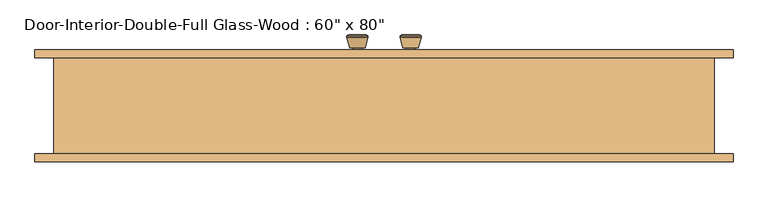
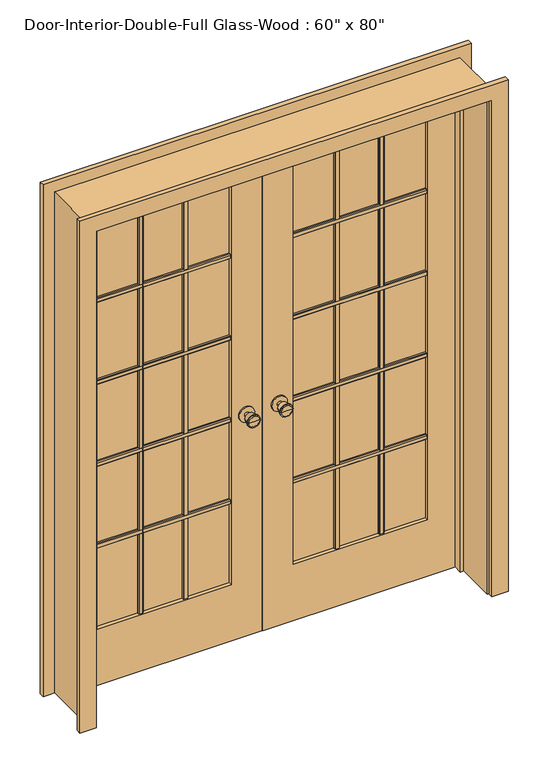
"""IFC4 building model written with IfcOpenShell, lengths in millimetres: door geometry."""

from ifc_helpers import new_model, si_unit, point, frame, frame_2d, origin, place, context, project, spatial, polyline, circle_curve, trimmed, segment, composite_curve, outline, extrude, faceted_brep, source, transform, mapped, element, save
from ifc_brep_helpers import plane_surface, cylinder_surface, revolved_surface, advanced_brep


def door_c5d3b7d7(model_context):
    return source(origin(), model_context, "Body", "SolidModel", [
        advanced_brep(
        [(-63.5, 117.125, 914.4), (-73.5, 117.125, 914.4), (-53.5, 117.125, 914.4), (-83.9758676, 166.125, 914.4), (-63.5, 166.125, 914.4), (-43.0241324, 166.125, 914.4), (-88.5, 164.2971319, 914.4), (-38.5, 164.2971319, 914.4), (-88.5, 160.8334537, 914.4), (-38.5, 160.8334537, 914.4), (-82.136236, 136.125, 914.4), (-44.863764, 136.125, 914.4), (-73.5, 136.125, 914.4), (-53.5, 136.125, 914.4)],
        [
            (0, 1),
            (1, 2, circle_curve(frame((-63.5, 117.125, 914.4), z_axis=(0.0, -1.0, 0.0), x_axis=(1.0, 0.0, 0.0)), 10.0)),
            (2, 0),
            (2, 1, circle_curve(frame((-63.5, 117.125, 914.4), z_axis=(0.0, -1.0, 0.0), x_axis=(1.0, 0.0, 0.0)), 10.0)),
            (3, 4),
            (4, 5),
            (5, 3, circle_curve(frame((-63.5, 166.125, 914.4), z_axis=(0.0, 1.0, 0.0), x_axis=(1.0, 0.0, 0.0)), 20.4758676)),
            (3, 5, circle_curve(frame((-63.5, 166.125, 914.4), z_axis=(0.0, 1.0, 0.0), x_axis=(1.0, 0.0, 0.0)), 20.4758676)),
            (6, 3),
            (5, 7),
            (7, 6, circle_curve(frame((-63.5, 164.2971319, 914.4), z_axis=(0.0, 1.0, 0.0), x_axis=(1.0, 0.0, 0.0)), 25.0)),
            (6, 7, circle_curve(frame((-63.5, 164.2971319, 914.4), z_axis=(0.0, 1.0, 0.0), x_axis=(1.0, 0.0, 0.0)), 25.0)),
            (8, 6),
            (7, 9),
            (9, 8, circle_curve(frame((-63.5, 160.8334537, 914.4), z_axis=(0.0, 1.0, 0.0), x_axis=(1.0, 0.0, 0.0)), 25.0)),
            (8, 9, circle_curve(frame((-63.5, 160.8334537, 914.4), z_axis=(0.0, 1.0, 0.0), x_axis=(1.0, 0.0, 0.0)), 25.0)),
            (10, 8),
            (9, 11),
            (11, 10, circle_curve(frame((-63.5, 136.125, 914.4), z_axis=(0.0, 1.0, 0.0), x_axis=(1.0, 0.0, 0.0)), 18.636236)),
            (10, 11, circle_curve(frame((-63.5, 136.125, 914.4), z_axis=(0.0, 1.0, 0.0), x_axis=(1.0, 0.0, 0.0)), 18.636236)),
            (12, 10),
            (11, 13),
            (13, 12, circle_curve(frame((-63.5, 136.125, 914.4), z_axis=(0.0, 1.0, 0.0), x_axis=(1.0, 0.0, 0.0)), 10.0)),
            (12, 13, circle_curve(frame((-63.5, 136.125, 914.4), z_axis=(0.0, 1.0, 0.0), x_axis=(1.0, 0.0, 0.0)), 10.0)),
            (1, 12),
            (13, 2),
        ],
        [
            plane_surface(frame((-63.5, 117.125, 914.4), z_axis=(0.0, -1.0, 0.0), x_axis=(1.0, 0.0, 0.0))),
            plane_surface(frame((-63.5, 166.125, 914.4), z_axis=(0.0, 1.0, 0.0), x_axis=(1.0, 0.0, 0.0))),
            revolved_surface(polyline([(-43.0241324, 166.125, 914.4), (-38.5, 164.2971319, 914.4)]), (-63.5, 117.125, 914.4), (0.0, -1.0, 0.0)),
            cylinder_surface(frame((-63.5, 117.125, 914.4), z_axis=(0.0, -1.0, 0.0), x_axis=(1.0, 0.0, 0.0)), 25.0),
            revolved_surface(polyline([(-38.5, 160.8334537, 914.4), (-44.863764, 136.125, 914.4)]), (-63.5, 117.125, 914.4), (0.0, -1.0, 0.0)),
            plane_surface(frame((-63.5, 136.125, 914.4), z_axis=(0.0, -1.0, 0.0), x_axis=(1.0, 0.0, 0.0))),
            cylinder_surface(frame((-63.5, 117.125, 914.4), z_axis=(0.0, -1.0, 0.0), x_axis=(1.0, 0.0, 0.0)), 10.0),
        ],
        [
            (0, [[1, 2, 3]]),
            (0, [[-3, 4, -1]]),
            (1, [[5, 6, 7]]),
            (1, [[-6, -5, 8]]),
            (2, [[9, -7, 10, 11]]),
            (2, [[-10, -8, -9, 12]]),
            (3, [[13, -11, 14, 15]]),
            (3, [[-14, -12, -13, 16]]),
            (4, [[17, -15, 18, 19]]),
            (4, [[-18, -16, -17, 20]]),
            (5, [[21, -19, 22, 23]]),
            (5, [[-22, -20, -21, 24]]),
            (6, [[25, -23, 26, -2]]),
            (6, [[-26, -24, -25, -4]]),
        ],
    ),
        extrude(outline(composite_curve([segment(trimmed(circle_curve(frame_2d((914.4, -63.5)), 30.0), [point((914.4, -33.5))], [point((914.4, -93.5))], False, "CARTESIAN"), True, "CONTINUOUS"), segment(trimmed(circle_curve(frame_2d((914.4, -63.5)), 30.0), [point((914.4, -93.5))], [point((914.4, -33.5))], False, "CARTESIAN"), True, "CONTINUOUS")], self_intersect=False)), frame((0.0, 111.125, 0.0), z_axis=(0.0, 1.0, 0.0), x_axis=(0.0, 0.0, 1.0)), (0.0, 0.0, 1.0), 6.0),
        advanced_brep(
        [(-63.5, 70.2, 914.4), (-53.5, 70.2, 914.4), (-73.5, 70.2, 914.4), (-83.9758676, 21.2, 914.4), (-43.0241324, 21.2, 914.4), (-63.5, 21.2, 914.4), (-88.5, 23.0278681, 914.4), (-38.5, 23.0278681, 914.4), (-88.5, 26.4915463, 914.4), (-38.5, 26.4915463, 914.4), (-82.136236, 51.2, 914.4), (-44.863764, 51.2, 914.4), (-73.5, 51.2, 914.4), (-53.5, 51.2, 914.4)],
        [
            (0, 1),
            (1, 2, circle_curve(frame((-63.5, 70.2, 914.4), z_axis=(0.0, 1.0, 0.0), x_axis=(1.0, 0.0, 0.0)), 10.0)),
            (2, 0),
            (2, 1, circle_curve(frame((-63.5, 70.2, 914.4), z_axis=(0.0, 1.0, 0.0), x_axis=(1.0, 0.0, 0.0)), 10.0)),
            (3, 4, circle_curve(frame((-63.5, 21.2, 914.4), z_axis=(0.0, -1.0, 0.0), x_axis=(1.0, 0.0, 0.0)), 20.4758676)),
            (4, 5),
            (5, 3),
            (4, 3, circle_curve(frame((-63.5, 21.2, 914.4), z_axis=(0.0, -1.0, 0.0), x_axis=(1.0, 0.0, 0.0)), 20.4758676)),
            (6, 7, circle_curve(frame((-63.5, 23.0278681, 914.4), z_axis=(0.0, -1.0, 0.0), x_axis=(1.0, 0.0, 0.0)), 25.0)),
            (7, 4),
            (3, 6),
            (7, 6, circle_curve(frame((-63.5, 23.0278681, 914.4), z_axis=(0.0, -1.0, 0.0), x_axis=(1.0, 0.0, 0.0)), 25.0)),
            (8, 9, circle_curve(frame((-63.5, 26.4915463, 914.4), z_axis=(0.0, -1.0, 0.0), x_axis=(1.0, 0.0, 0.0)), 25.0)),
            (9, 7),
            (6, 8),
            (9, 8, circle_curve(frame((-63.5, 26.4915463, 914.4), z_axis=(0.0, -1.0, 0.0), x_axis=(1.0, 0.0, 0.0)), 25.0)),
            (10, 11, circle_curve(frame((-63.5, 51.2, 914.4), z_axis=(0.0, -1.0, 0.0), x_axis=(1.0, 0.0, 0.0)), 18.636236)),
            (11, 9),
            (8, 10),
            (11, 10, circle_curve(frame((-63.5, 51.2, 914.4), z_axis=(0.0, -1.0, 0.0), x_axis=(1.0, 0.0, 0.0)), 18.636236)),
            (12, 13, circle_curve(frame((-63.5, 51.2, 914.4), z_axis=(0.0, -1.0, 0.0), x_axis=(1.0, 0.0, 0.0)), 10.0)),
            (13, 11),
            (10, 12),
            (13, 12, circle_curve(frame((-63.5, 51.2, 914.4), z_axis=(0.0, -1.0, 0.0), x_axis=(1.0, 0.0, 0.0)), 10.0)),
            (1, 13),
            (12, 2),
        ],
        [
            plane_surface(frame((-63.5, 70.2, 914.4), z_axis=(0.0, 1.0, 0.0), x_axis=(1.0, 0.0, 0.0))),
            plane_surface(frame((-63.5, 21.2, 914.4), z_axis=(0.0, -1.0, 0.0), x_axis=(1.0, 0.0, 0.0))),
            revolved_surface(polyline([(-43.0241324, 21.2, 914.4), (-38.5, 23.0278681, 914.4)]), (-63.5, 70.2, 914.4), (0.0, 1.0, 0.0)),
            cylinder_surface(frame((-63.5, 70.2, 914.4), z_axis=(0.0, 1.0, 0.0), x_axis=(1.0, 0.0, 0.0)), 25.0),
            revolved_surface(polyline([(-38.5, 26.4915463, 914.4), (-44.863764, 51.2, 914.4)]), (-63.5, 70.2, 914.4), (0.0, 1.0, 0.0)),
            plane_surface(frame((-63.5, 51.2, 914.4), z_axis=(0.0, 1.0, 0.0), x_axis=(1.0, 0.0, 0.0))),
            cylinder_surface(frame((-63.5, 70.2, 914.4), z_axis=(0.0, 1.0, 0.0), x_axis=(1.0, 0.0, 0.0)), 10.0),
        ],
        [
            (0, [[1, 2, 3]]),
            (0, [[-3, 4, -1]]),
            (1, [[5, 6, 7]]),
            (1, [[8, -7, -6]]),
            (2, [[9, 10, -5, 11]]),
            (2, [[12, -11, -8, -10]]),
            (3, [[13, 14, -9, 15]]),
            (3, [[16, -15, -12, -14]]),
            (4, [[17, 18, -13, 19]]),
            (4, [[20, -19, -16, -18]]),
            (5, [[21, 22, -17, 23]]),
            (5, [[24, -23, -20, -22]]),
            (6, [[-2, 25, -21, 26]]),
            (6, [[-4, -26, -24, -25]]),
        ],
    ),
        extrude(outline(composite_curve([segment(trimmed(circle_curve(frame_2d((914.4, -63.5)), 30.0), [point((914.4, -33.5))], [point((914.4, -93.5))], False, "CARTESIAN"), True, "CONTINUOUS"), segment(trimmed(circle_curve(frame_2d((914.4, -63.5)), 30.0), [point((914.4, -93.5))], [point((914.4, -33.5))], False, "CARTESIAN"), True, "CONTINUOUS")], self_intersect=False)), frame((0.0, 70.2, 0.0), z_axis=(0.0, 1.0, 0.0), x_axis=(0.0, 0.0, 1.0)), (0.0, 0.0, 1.0), 6.0),
        extrude(outline(polyline([(90.17, 1586.23), (90.17, 1567.18), (83.82, 1567.18), (80.645, 1570.355), (80.645, 1583.055), (83.82, 1586.23), (90.17, 1586.23)])), frame((120.65, 0.0, 0.0), z_axis=(1.0, 0.0, 0.0), x_axis=(0.0, 1.0, 0.0)), (0.0, 0.0, 1.0), 520.7),
        extrude(outline(polyline([(90.17, 1249.9975), (90.17, 1230.9475), (83.82, 1230.9475), (80.645, 1234.1225), (80.645, 1246.8225), (83.82, 1249.9975), (90.17, 1249.9975)])), frame((120.65, 0.0, 0.0), z_axis=(1.0, 0.0, 0.0), x_axis=(0.0, 1.0, 0.0)), (0.0, 0.0, 1.0), 520.7),
        extrude(outline(polyline([(90.17, 913.765), (90.17, 894.715), (83.82, 894.715), (80.645, 897.89), (80.645, 910.59), (83.82, 913.765), (90.17, 913.765)])), frame((120.65, 0.0, 0.0), z_axis=(1.0, 0.0, 0.0), x_axis=(0.0, 1.0, 0.0)), (0.0, 0.0, 1.0), 520.7),
        extrude(outline(polyline([(90.17, 577.5325), (90.17, 558.4825), (83.82, 558.4825), (80.645, 561.6575), (80.645, 574.3575), (83.82, 577.5325), (90.17, 577.5325)])), frame((120.65, 0.0, 0.0), z_axis=(1.0, 0.0, 0.0), x_axis=(0.0, 1.0, 0.0)), (0.0, 0.0, 1.0), 520.7),
        extrude(outline(polyline([(458.2583333, 90.17), (477.3083333, 90.17), (477.3083333, 83.82), (474.1333333, 80.645), (461.4333333, 80.645), (458.2583333, 83.82), (458.2583333, 90.17)])), frame((0.0, 0.0, 231.775), z_axis=(0.0, 0.0, 1.0), x_axis=(1.0, 0.0, 0.0)), (0.0, 0.0, 1.0), 1681.1625),
        extrude(outline(polyline([(284.6916667, 90.17), (303.7416667, 90.17), (303.7416667, 83.82), (300.5666667, 80.645), (287.8666667, 80.645), (284.6916667, 83.82), (284.6916667, 90.17)])), frame((0.0, 0.0, 231.775), z_axis=(0.0, 0.0, 1.0), x_axis=(1.0, 0.0, 0.0)), (0.0, 0.0, 1.0), 1681.1625),
        extrude(outline(polyline([(97.155, 1586.23), (103.505, 1586.23), (106.68, 1583.055), (106.68, 1570.355), (103.505, 1567.18), (97.155, 1567.18), (97.155, 1586.23)])), frame((-641.35, 0.0, 0.0), z_axis=(1.0, 0.0, 0.0), x_axis=(0.0, 1.0, 0.0)), (0.0, 0.0, 1.0), 520.7),
        extrude(outline(polyline([(97.155, 1249.9975), (103.505, 1249.9975), (106.68, 1246.8225), (106.68, 1234.1225), (103.505, 1230.9475), (97.155, 1230.9475), (97.155, 1249.9975)])), frame((-641.35, 0.0, 0.0), z_axis=(1.0, 0.0, 0.0), x_axis=(0.0, 1.0, 0.0)), (0.0, 0.0, 1.0), 520.7),
        extrude(outline(polyline([(97.155, 913.765), (103.505, 913.765), (106.68, 910.59), (106.68, 897.89), (103.505, 894.715), (97.155, 894.715), (97.155, 913.765)])), frame((-641.35, 0.0, 0.0), z_axis=(1.0, 0.0, 0.0), x_axis=(0.0, 1.0, 0.0)), (0.0, 0.0, 1.0), 520.7),
        extrude(outline(polyline([(97.155, 577.5325), (103.505, 577.5325), (106.68, 574.3575), (106.68, 561.6575), (103.505, 558.4825), (97.155, 558.4825), (97.155, 577.5325)])), frame((-641.35, 0.0, 0.0), z_axis=(1.0, 0.0, 0.0), x_axis=(0.0, 1.0, 0.0)), (0.0, 0.0, 1.0), 520.7),
        extrude(outline(polyline([(-303.7416667, 97.155), (-303.7416667, 103.505), (-300.5666667, 106.68), (-287.8666667, 106.68), (-284.6916667, 103.505), (-284.6916667, 97.155), (-303.7416667, 97.155)])), frame((0.0, 0.0, 231.775), z_axis=(0.0, 0.0, 1.0), x_axis=(1.0, 0.0, 0.0)), (0.0, 0.0, 1.0), 1681.1625),
        extrude(outline(polyline([(-477.3083333, 97.155), (-477.3083333, 103.505), (-474.1333333, 106.68), (-461.4333333, 106.68), (-458.2583333, 103.505), (-458.2583333, 97.155), (-477.3083333, 97.155)])), frame((0.0, 0.0, 231.775), z_axis=(0.0, 0.0, 1.0), x_axis=(1.0, 0.0, 0.0)), (0.0, 0.0, 1.0), 1681.1625),
        extrude(outline(polyline([(97.155, 1586.23), (103.505, 1586.23), (106.68, 1583.055), (106.68, 1570.355), (103.505, 1567.18), (97.155, 1567.18), (97.155, 1586.23)])), frame((120.65, 0.0, 0.0), z_axis=(1.0, 0.0, 0.0), x_axis=(0.0, 1.0, 0.0)), (0.0, 0.0, 1.0), 520.7),
        extrude(outline(polyline([(97.155, 1249.9975), (103.505, 1249.9975), (106.68, 1246.8225), (106.68, 1234.1225), (103.505, 1230.9475), (97.155, 1230.9475), (97.155, 1249.9975)])), frame((120.65, 0.0, 0.0), z_axis=(1.0, 0.0, 0.0), x_axis=(0.0, 1.0, 0.0)), (0.0, 0.0, 1.0), 520.7),
        extrude(outline(polyline([(97.155, 913.765), (103.505, 913.765), (106.68, 910.59), (106.68, 897.89), (103.505, 894.715), (97.155, 894.715), (97.155, 913.765)])), frame((120.65, 0.0, 0.0), z_axis=(1.0, 0.0, 0.0), x_axis=(0.0, 1.0, 0.0)), (0.0, 0.0, 1.0), 520.7),
        extrude(outline(polyline([(97.155, 577.5325), (103.505, 577.5325), (106.68, 574.3575), (106.68, 561.6575), (103.505, 558.4825), (97.155, 558.4825), (97.155, 577.5325)])), frame((120.65, 0.0, 0.0), z_axis=(1.0, 0.0, 0.0), x_axis=(0.0, 1.0, 0.0)), (0.0, 0.0, 1.0), 520.7),
        extrude(outline(polyline([(458.2583333, 97.155), (458.2583333, 103.505), (461.4333333, 106.68), (474.1333333, 106.68), (477.3083333, 103.505), (477.3083333, 97.155), (458.2583333, 97.155)])), frame((0.0, 0.0, 231.775), z_axis=(0.0, 0.0, 1.0), x_axis=(1.0, 0.0, 0.0)), (0.0, 0.0, 1.0), 1681.1625),
        extrude(outline(polyline([(284.6916667, 97.155), (284.6916667, 103.505), (287.8666667, 106.68), (300.5666667, 106.68), (303.7416667, 103.505), (303.7416667, 97.155), (284.6916667, 97.155)])), frame((0.0, 0.0, 231.775), z_axis=(0.0, 0.0, 1.0), x_axis=(1.0, 0.0, 0.0)), (0.0, 0.0, 1.0), 1681.1625),
        extrude(outline(polyline([(90.17, 1586.23), (90.17, 1567.18), (83.82, 1567.18), (80.645, 1570.355), (80.645, 1583.055), (83.82, 1586.23), (90.17, 1586.23)])), frame((-641.35, 0.0, 0.0), z_axis=(1.0, 0.0, 0.0), x_axis=(0.0, 1.0, 0.0)), (0.0, 0.0, 1.0), 520.7),
        extrude(outline(polyline([(90.17, 1249.9975), (90.17, 1230.9475), (83.82, 1230.9475), (80.645, 1234.1225), (80.645, 1246.8225), (83.82, 1249.9975), (90.17, 1249.9975)])), frame((-641.35, 0.0, 0.0), z_axis=(1.0, 0.0, 0.0), x_axis=(0.0, 1.0, 0.0)), (0.0, 0.0, 1.0), 520.7),
        extrude(outline(polyline([(90.17, 913.765), (90.17, 894.715), (83.82, 894.715), (80.645, 897.89), (80.645, 910.59), (83.82, 913.765), (90.17, 913.765)])), frame((-641.35, 0.0, 0.0), z_axis=(1.0, 0.0, 0.0), x_axis=(0.0, 1.0, 0.0)), (0.0, 0.0, 1.0), 520.7),
        extrude(outline(polyline([(90.17, 577.5325), (90.17, 558.4825), (83.82, 558.4825), (80.645, 561.6575), (80.645, 574.3575), (83.82, 577.5325), (90.17, 577.5325)])), frame((-641.35, 0.0, 0.0), z_axis=(1.0, 0.0, 0.0), x_axis=(0.0, 1.0, 0.0)), (0.0, 0.0, 1.0), 520.7),
        extrude(outline(polyline([(-303.7416667, 90.17), (-284.6916667, 90.17), (-284.6916667, 83.82), (-287.8666667, 80.645), (-300.5666667, 80.645), (-303.7416667, 83.82), (-303.7416667, 90.17)])), frame((0.0, 0.0, 231.775), z_axis=(0.0, 0.0, 1.0), x_axis=(1.0, 0.0, 0.0)), (0.0, 0.0, 1.0), 1681.1625),
        extrude(outline(polyline([(-477.3083333, 90.17), (-458.2583333, 90.17), (-458.2583333, 83.82), (-461.4333333, 80.645), (-474.1333333, 80.645), (-477.3083333, 83.82), (-477.3083333, 90.17)])), frame((0.0, 0.0, 231.775), z_axis=(0.0, 0.0, 1.0), x_axis=(1.0, 0.0, 0.0)), (0.0, 0.0, 1.0), 1681.1625),
        advanced_brep(
        [(63.5, 70.2, 914.4), (73.5, 70.2, 914.4), (53.5, 70.2, 914.4), (83.9758676, 21.2, 914.4), (63.5, 21.2, 914.4), (43.0241324, 21.2, 914.4), (88.5, 23.0278681, 914.4), (38.5, 23.0278681, 914.4), (88.5, 26.4915463, 914.4), (38.5, 26.4915463, 914.4), (82.136236, 51.2, 914.4), (44.863764, 51.2, 914.4), (73.5, 51.2, 914.4), (53.5, 51.2, 914.4)],
        [
            (0, 1),
            (1, 2, circle_curve(frame((63.5, 70.2, 914.4), z_axis=(0.0, 1.0, 0.0), x_axis=(-1.0, 0.0, 0.0)), 10.0)),
            (2, 0),
            (2, 1, circle_curve(frame((63.5, 70.2, 914.4), z_axis=(0.0, 1.0, 0.0), x_axis=(-1.0, 0.0, 0.0)), 10.0)),
            (3, 4),
            (4, 5),
            (5, 3, circle_curve(frame((63.5, 21.2, 914.4), z_axis=(0.0, -1.0, 0.0), x_axis=(-1.0, 0.0, 0.0)), 20.4758676)),
            (3, 5, circle_curve(frame((63.5, 21.2, 914.4), z_axis=(0.0, -1.0, 0.0), x_axis=(-1.0, 0.0, 0.0)), 20.4758676)),
            (6, 3),
            (5, 7),
            (7, 6, circle_curve(frame((63.5, 23.0278681, 914.4), z_axis=(0.0, -1.0, 0.0), x_axis=(-1.0, 0.0, 0.0)), 25.0)),
            (6, 7, circle_curve(frame((63.5, 23.0278681, 914.4), z_axis=(0.0, -1.0, 0.0), x_axis=(-1.0, 0.0, 0.0)), 25.0)),
            (8, 6),
            (7, 9),
            (9, 8, circle_curve(frame((63.5, 26.4915463, 914.4), z_axis=(0.0, -1.0, 0.0), x_axis=(-1.0, 0.0, 0.0)), 25.0)),
            (8, 9, circle_curve(frame((63.5, 26.4915463, 914.4), z_axis=(0.0, -1.0, 0.0), x_axis=(-1.0, 0.0, 0.0)), 25.0)),
            (10, 8),
            (9, 11),
            (11, 10, circle_curve(frame((63.5, 51.2, 914.4), z_axis=(0.0, -1.0, 0.0), x_axis=(-1.0, 0.0, 0.0)), 18.636236)),
            (10, 11, circle_curve(frame((63.5, 51.2, 914.4), z_axis=(0.0, -1.0, 0.0), x_axis=(-1.0, 0.0, 0.0)), 18.636236)),
            (12, 10),
            (11, 13),
            (13, 12, circle_curve(frame((63.5, 51.2, 914.4), z_axis=(0.0, -1.0, 0.0), x_axis=(-1.0, 0.0, 0.0)), 10.0)),
            (12, 13, circle_curve(frame((63.5, 51.2, 914.4), z_axis=(0.0, -1.0, 0.0), x_axis=(-1.0, 0.0, 0.0)), 10.0)),
            (1, 12),
            (13, 2),
        ],
        [
            plane_surface(frame((63.5, 70.2, 914.4), z_axis=(0.0, 1.0, 0.0), x_axis=(-1.0, 0.0, 0.0))),
            plane_surface(frame((63.5, 21.2, 914.4), z_axis=(0.0, -1.0, 0.0), x_axis=(-1.0, 0.0, 0.0))),
            revolved_surface(polyline([(43.0241324, 21.2, 914.4), (38.5, 23.0278681, 914.4)]), (63.5, 70.2, 914.4), (0.0, 1.0, 0.0)),
            cylinder_surface(frame((63.5, 70.2, 914.4), z_axis=(0.0, 1.0, 0.0), x_axis=(-1.0, 0.0, 0.0)), 25.0),
            revolved_surface(polyline([(38.5, 26.4915463, 914.4), (44.863764, 51.2, 914.4)]), (63.5, 70.2, 914.4), (0.0, 1.0, 0.0)),
            plane_surface(frame((63.5, 51.2, 914.4), z_axis=(0.0, 1.0, 0.0), x_axis=(-1.0, 0.0, 0.0))),
            cylinder_surface(frame((63.5, 70.2, 914.4), z_axis=(0.0, 1.0, 0.0), x_axis=(-1.0, 0.0, 0.0)), 10.0),
        ],
        [
            (0, [[1, 2, 3]]),
            (0, [[-3, 4, -1]]),
            (1, [[5, 6, 7]]),
            (1, [[-6, -5, 8]]),
            (2, [[9, -7, 10, 11]]),
            (2, [[-10, -8, -9, 12]]),
            (3, [[13, -11, 14, 15]]),
            (3, [[-14, -12, -13, 16]]),
            (4, [[17, -15, 18, 19]]),
            (4, [[-18, -16, -17, 20]]),
            (5, [[21, -19, 22, 23]]),
            (5, [[-22, -20, -21, 24]]),
            (6, [[25, -23, 26, -2]]),
            (6, [[-26, -24, -25, -4]]),
        ],
    ),
        extrude(outline(composite_curve([segment(trimmed(circle_curve(frame_2d((914.4, 63.5)), 30.0), [point((914.4, 33.5))], [point((914.4, 93.5))], False, "CARTESIAN"), True, "CONTINUOUS"), segment(trimmed(circle_curve(frame_2d((914.4, 63.5)), 30.0), [point((914.4, 93.5))], [point((914.4, 33.5))], False, "CARTESIAN"), True, "CONTINUOUS")], self_intersect=False)), frame((0.0, 70.2, 0.0), z_axis=(0.0, 1.0, 0.0), x_axis=(0.0, 0.0, 1.0)), (0.0, 0.0, 1.0), 6.0),
        advanced_brep(
        [(63.5, 117.125, 914.4), (53.5, 117.125, 914.4), (73.5, 117.125, 914.4), (83.9758676, 166.125, 914.4), (43.0241324, 166.125, 914.4), (63.5, 166.125, 914.4), (88.5, 164.2971319, 914.4), (38.5, 164.2971319, 914.4), (88.5, 160.8334537, 914.4), (38.5, 160.8334537, 914.4), (82.136236, 136.125, 914.4), (44.863764, 136.125, 914.4), (73.5, 136.125, 914.4), (53.5, 136.125, 914.4)],
        [
            (0, 1),
            (1, 2, circle_curve(frame((63.5, 117.125, 914.4), z_axis=(0.0, -1.0, 0.0), x_axis=(-1.0, 0.0, 0.0)), 10.0)),
            (2, 0),
            (2, 1, circle_curve(frame((63.5, 117.125, 914.4), z_axis=(0.0, -1.0, 0.0), x_axis=(-1.0, 0.0, 0.0)), 10.0)),
            (3, 4, circle_curve(frame((63.5, 166.125, 914.4), z_axis=(0.0, 1.0, 0.0), x_axis=(-1.0, 0.0, 0.0)), 20.4758676)),
            (4, 5),
            (5, 3),
            (4, 3, circle_curve(frame((63.5, 166.125, 914.4), z_axis=(0.0, 1.0, 0.0), x_axis=(-1.0, 0.0, 0.0)), 20.4758676)),
            (6, 7, circle_curve(frame((63.5, 164.2971319, 914.4), z_axis=(0.0, 1.0, 0.0), x_axis=(-1.0, 0.0, 0.0)), 25.0)),
            (7, 4),
            (3, 6),
            (7, 6, circle_curve(frame((63.5, 164.2971319, 914.4), z_axis=(0.0, 1.0, 0.0), x_axis=(-1.0, 0.0, 0.0)), 25.0)),
            (8, 9, circle_curve(frame((63.5, 160.8334537, 914.4), z_axis=(0.0, 1.0, 0.0), x_axis=(-1.0, 0.0, 0.0)), 25.0)),
            (9, 7),
            (6, 8),
            (9, 8, circle_curve(frame((63.5, 160.8334537, 914.4), z_axis=(0.0, 1.0, 0.0), x_axis=(-1.0, 0.0, 0.0)), 25.0)),
            (10, 11, circle_curve(frame((63.5, 136.125, 914.4), z_axis=(0.0, 1.0, 0.0), x_axis=(-1.0, 0.0, 0.0)), 18.636236)),
            (11, 9),
            (8, 10),
            (11, 10, circle_curve(frame((63.5, 136.125, 914.4), z_axis=(0.0, 1.0, 0.0), x_axis=(-1.0, 0.0, 0.0)), 18.636236)),
            (12, 13, circle_curve(frame((63.5, 136.125, 914.4), z_axis=(0.0, 1.0, 0.0), x_axis=(-1.0, 0.0, 0.0)), 10.0)),
            (13, 11),
            (10, 12),
            (13, 12, circle_curve(frame((63.5, 136.125, 914.4), z_axis=(0.0, 1.0, 0.0), x_axis=(-1.0, 0.0, 0.0)), 10.0)),
            (1, 13),
            (12, 2),
        ],
        [
            plane_surface(frame((63.5, 117.125, 914.4), z_axis=(0.0, -1.0, 0.0), x_axis=(-1.0, 0.0, 0.0))),
            plane_surface(frame((63.5, 166.125, 914.4), z_axis=(0.0, 1.0, 0.0), x_axis=(-1.0, 0.0, 0.0))),
            revolved_surface(polyline([(43.0241324, 166.125, 914.4), (38.5, 164.2971319, 914.4)]), (63.5, 117.125, 914.4), (0.0, -1.0, 0.0)),
            cylinder_surface(frame((63.5, 117.125, 914.4), z_axis=(0.0, -1.0, 0.0), x_axis=(-1.0, 0.0, 0.0)), 25.0),
            revolved_surface(polyline([(38.5, 160.8334537, 914.4), (44.863764, 136.125, 914.4)]), (63.5, 117.125, 914.4), (0.0, -1.0, 0.0)),
            plane_surface(frame((63.5, 136.125, 914.4), z_axis=(0.0, -1.0, 0.0), x_axis=(-1.0, 0.0, 0.0))),
            cylinder_surface(frame((63.5, 117.125, 914.4), z_axis=(0.0, -1.0, 0.0), x_axis=(-1.0, 0.0, 0.0)), 10.0),
        ],
        [
            (0, [[1, 2, 3]]),
            (0, [[-3, 4, -1]]),
            (1, [[5, 6, 7]]),
            (1, [[8, -7, -6]]),
            (2, [[9, 10, -5, 11]]),
            (2, [[12, -11, -8, -10]]),
            (3, [[13, 14, -9, 15]]),
            (3, [[16, -15, -12, -14]]),
            (4, [[17, 18, -13, 19]]),
            (4, [[20, -19, -16, -18]]),
            (5, [[21, 22, -17, 23]]),
            (5, [[24, -23, -20, -22]]),
            (6, [[-2, 25, -21, 26]]),
            (6, [[-4, -26, -24, -25]]),
        ],
    ),
        extrude(outline(composite_curve([segment(trimmed(circle_curve(frame_2d((914.4, 63.5)), 30.0), [point((914.4, 33.5))], [point((914.4, 93.5))], False, "CARTESIAN"), True, "CONTINUOUS"), segment(trimmed(circle_curve(frame_2d((914.4, 63.5)), 30.0), [point((914.4, 93.5))], [point((914.4, 33.5))], False, "CARTESIAN"), True, "CONTINUOUS")], self_intersect=False)), frame((0.0, 111.125, 0.0), z_axis=(0.0, 1.0, 0.0), x_axis=(0.0, 0.0, 1.0)), (0.0, 0.0, 1.0), 6.0),
        extrude(outline(polyline([(0.0, 768.35), (0.0, 831.85), (2101.85, 831.85), (2101.85, -831.85), (0.0, -831.85), (0.0, -768.35), (2038.35, -768.35), (2038.35, 768.35), (0.0, 768.35)])), frame((0.0, -136.525, 0.0), z_axis=(0.0, 1.0, 0.0), x_axis=(0.0, 0.0, 1.0)), (0.0, 0.0, 1.0), 19.05),
        extrude(outline(polyline([(0.0, 768.35), (0.0, 831.85), (2101.85, 831.85), (2101.85, -831.85), (0.0, -831.85), (0.0, -768.35), (2038.35, -768.35), (2038.35, 768.35), (0.0, 768.35)])), frame((0.0, 111.125, 0.0), z_axis=(0.0, 1.0, 0.0), x_axis=(0.0, 0.0, 1.0)), (0.0, 0.0, 1.0), 19.05),
        faceted_brep([(787.4, 111.125, 0.0), (787.4, -117.475, 0.0), (762.0, -117.475, 0.0), (762.0, 41.275, 0.0), (749.3, 41.275, 0.0), (749.3, 76.2, 0.0), (762.0, 76.2, 0.0), (762.0, 111.125, 0.0), (787.4, 111.125, 2057.4), (787.4, -117.475, 2057.4), (-787.4, -117.475, 2057.4), (-787.4, -117.475, 0.0), (-762.0, -117.475, 0.0), (-762.0, -117.475, 2032.0), (762.0, -117.475, 2032.0), (762.0, 41.275, 2032.0), (-762.0, 41.275, 2032.0), (-762.0, 41.275, 0.0), (-749.3, 41.275, 0.0), (-749.3, 41.275, 2019.3), (749.3, 41.275, 2019.3), (749.3, 76.2, 2019.3), (1.5875, 76.2, 2019.3), (-1.6019111, 76.2, 2019.3), (-749.3, 76.2, 2019.3), (-749.3, 76.2, 0.0), (-762.0, 76.2, 0.0), (-762.0, 76.2, 2032.0), (-1.6019111, 76.2, 2032.0), (1.5875, 76.2, 2032.0), (762.0, 76.2, 2032.0), (762.0, 111.125, 2032.0), (1.5875, 111.125, 2032.0), (-1.6019111, 111.125, 2032.0), (-762.0, 111.125, 2032.0), (-762.0, 111.125, 0.0), (-787.4, 111.125, 0.0), (-787.4, 111.125, 2057.4)], [[[0, 1, 2, 3, 4, 5, 6, 7]], [[1, 0, 8, 9]], [[2, 1, 9, 10, 11, 12, 13, 14]], [[3, 2, 14, 15]], [[4, 3, 15, 16, 17, 18, 19, 20]], [[5, 4, 20, 21]], [[6, 5, 21, 22, 23, 24, 25, 26, 27, 28, 29, 30]], [[7, 6, 30, 31]], [[0, 7, 31, 32, 33, 34, 35, 36, 37, 8]], [[9, 8, 37, 10]], [[14, 13, 16, 15]], [[20, 19, 24, 23, 22, 21]], [[31, 30, 29, 28, 27, 34, 33, 32]], [[12, 11, 36, 35, 26, 25, 18, 17]], [[11, 10, 37, 36]], [[13, 12, 17, 16]], [[19, 18, 25, 24]], [[27, 26, 35, 34]]]),
        extrude(outline(polyline([(2032.0, -762.0), (0.0, -762.0), (0.0, -1.6019111), (2032.0, -1.6019111), (2032.0, -762.0)]), holes=[polyline([(231.775, -641.35), (1912.9375, -641.35), (1912.9375, -120.65), (231.775, -120.65), (231.775, -641.35)])]), frame((0.0, 76.2, 0.0), z_axis=(0.0, 1.0, 0.0), x_axis=(0.0, 0.0, 1.0)), (0.0, 0.0, 1.0), 34.925),
        extrude(outline(polyline([(0.0, 762.0), (2032.0, 762.0), (2032.0, 1.5875), (0.0, 1.5875), (0.0, 762.0)]), holes=[polyline([(1912.9375, 120.65), (1912.9375, 641.35), (231.775, 641.35), (231.775, 120.65), (1912.9375, 120.65)])]), frame((0.0, 76.2, 0.0), z_axis=(0.0, 1.0, 0.0), x_axis=(0.0, 0.0, 1.0)), (0.0, 0.0, 1.0), 34.925),
        extrude(outline(polyline([(641.35, 90.17), (120.65, 90.17), (120.65, 97.155), (641.35, 97.155), (641.35, 90.17)])), frame((0.0, 0.0, 231.775), z_axis=(0.0, 0.0, 1.0), x_axis=(1.0, 0.0, 0.0)), (0.0, 0.0, 1.0), 1681.1625),
        extrude(outline(polyline([(-120.65, 90.17), (-641.35, 90.17), (-641.35, 97.155), (-120.65, 97.155), (-120.65, 90.17)])), frame((0.0, 0.0, 231.775), z_axis=(0.0, 0.0, 1.0), x_axis=(1.0, 0.0, 0.0)), (0.0, 0.0, 1.0), 1681.1625),
    ])


if __name__ == "__main__":
    model = new_model("IFC4")
    model_context = context("Model", 3, world=origin())
    ifc_project = project(units=[si_unit("LENGTHUNIT", "METRE", prefix="MILLI")], contexts=[model_context])
    site = spatial("IfcSite", under=ifc_project)
    building = spatial("IfcBuilding", under=site)
    placement = place(None, origin())
    door_shape = door_c5d3b7d7(model_context)
    element("IfcDoor", 1, ObjectType="Door-Interior-Double-Full Glass-Wood : 60\" x 80\"", at=placement, inside=building, context=model_context, shape_type="MappedRepresentation", body=[
        mapped(door_shape, transform((0.0, 0.0, 0.0), x_axis=(1.0, 0.0, 0.0), y_axis=(0.0, 1.0, 0.0), z_axis=(0.0, 0.0, 1.0))),
    ])
    save(model, "model.ifc")

# Revit data of these elements
# Type "Door-Interior-Double-Full Glass-Wood : 60\" x 80\""
#   Type Mark = "8"
#   Assembly Code = "C1020300"
#   Analytic Construction = "French door, wood frame with single glass"
#   Top Rail = 0' - 4 11/16"
#   Thickness = 0' - 1 3/8"
#   Thermal Resistance (R) = 1.0696 (h·ft²·°F)/BTU
#   Swing Angle [instance default] = 90.00°
#   Stiles = 0' - 4 3/4"
#   Rough Width = 5' - 2"
#   Rough Height = 6' - 9"
#   Panel Width = 2' - 6"
#   Height = 6' - 8"
#   Width = 5' - 0"
#   Heat Transfer Coefficient (U) = 0.9350 BTU/(h·ft²·°F)
#   Bottom Rail = 0' - 9 1/8"
#   Show Grill [instance default] = yes
#   Trim Material = Cherry
#   Panel Material = Cherry
#   Frame Material = Cherry
#   Door Handle Material = Aluminum
#   Visual Light Transmittance = 0
#   Solar Heat Gain Coefficient = 0
#   Wall Closure = (empty or 0)
#   Function = (empty or 0)
# Element 1 (IfcDoor, "Door-Interior-Double-Full Glass-Wood : 60\" x 80\"")
#   Materials on its faces: "Cherry", "Aluminum", "Glass"
# Materials
#   "Cherry": class "Wood", colour RGB 226 177 128, transparency 0, Description = "Prunus Serotina", Cost = 0
#   "Aluminum": class "Metal", colour RGB 247 247 247, transparency 0, Description = "Aluminum 6061", Cost = 0
#   "Glass": class "Glass", colour RGB 0 128 192, transparency 0.75, Description = "Soda Lime Glass", Cost = 0
